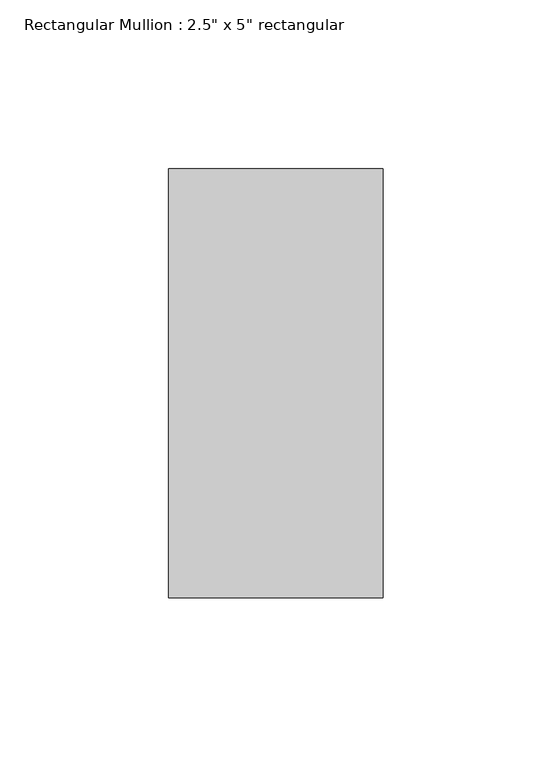
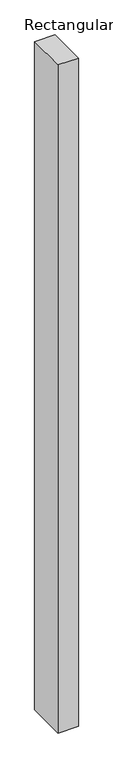
"""IFC4 building model written with IfcOpenShell, lengths in millimetres: member geometry."""

from ifc_helpers import new_model, si_unit, frame, origin, place, context, project, spatial, polyline, outline, extrude, source, transform, mapped, element, save


def member_04cfd63f(model_context):
    return source(origin(), model_context, "Body", "SweptSolid", [
        extrude(outline(polyline([(0.0, 63.5), (0.0, -63.5), (-63.5, -63.5), (-63.5, 63.5), (0.0, 63.5)])), frame((0.0, 0.0, -2214.4457658), z_axis=(0.0, 0.0, 1.0), x_axis=(1.0, 0.0, 0.0)), (0.0, 0.0, 1.0), 2214.4457658),
    ])


if __name__ == "__main__":
    model = new_model("IFC4")
    model_context = context("Model", 3, world=origin())
    ifc_project = project(units=[si_unit("LENGTHUNIT", "METRE", prefix="MILLI")], contexts=[model_context])
    site = spatial("IfcSite", under=ifc_project)
    building = spatial("IfcBuilding", under=site)
    placement = place(None, origin())
    member_shape = member_04cfd63f(model_context)
    element("IfcMember", 1, ObjectType="Rectangular Mullion : 2.5\" x 5\" rectangular", at=placement, inside=building, context=model_context, shape_type="MappedRepresentation", body=[
        mapped(member_shape, transform((0.0, 0.0, 0.0), x_axis=(1.0, 0.0, 0.0), y_axis=(0.0, 1.0, 0.0), z_axis=(0.0, 0.0, 1.0))),
    ])
    save(model, "model.ifc")

# Revit data of these elements
# Type "Rectangular Mullion : 2.5\" x 5\" rectangular"
#   built-in parameter 1007304 = 0.416667 (stored number, unit not read)
#   built-in parameter 1007301 = 0.104167 (stored number, unit not read)
#   built-in parameter 1007300 = 0.104167 (stored number, unit not read)
# Element 1 (IfcMember, "Rectangular Mullion : 2.5\" x 5\" rectangular")
#   Materials on its faces: "Aluminum"
# Materials
#   "Aluminum": class "Metal", colour RGB 247 247 247, transparency 0, Description = "Aluminum 6061", Cost = 0
